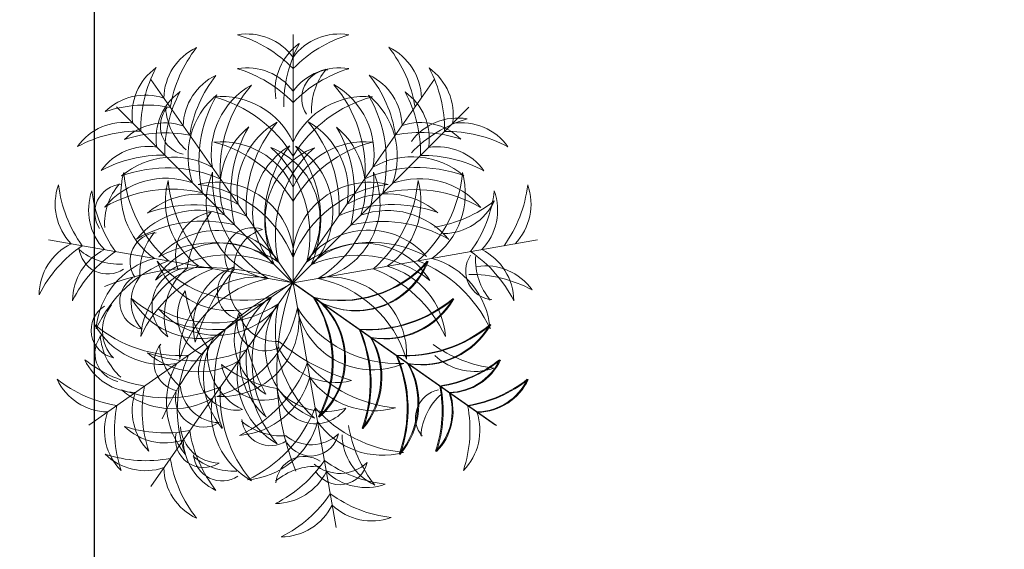
# Model space of a CAD drawing. Units: inches. Extents: x -48 to 50072, y 0 to 21068.
# Tile 10 of 75: x 212 to 263, y 278 to 305. Entities that reach past the tile are written whole.
import ezdxf

# ---------------------------------------------------------------- set-up
doc = ezdxf.new("R2010")
doc.units = ezdxf.units.IN
doc.header["$MEASUREMENT"] = 0
doc.layers.add('A-ANNO-DIMS', color=2, linetype='Continuous', lineweight=18)
doc.layers.add('L-PLNT', color=94, linetype='Continuous', lineweight=13)
doc.styles.get("Standard").update_dxf_attribs({"font": 'arial.ttf'})
doc.dimstyles.get("Standard").update_dxf_attribs({"dimtxt": 8, "dimasz": 0.18, "dimexe": 0.18, "dimexo": 0.0625, "dimgap": 0.09, "dimtad": 0, "dimtih": 1, "dimtoh": 1, "dimdec": 1, "dimzin": 0, "dimdsep": 46, "dimlunit": 4, "dimtxsty": 'Standard', "dimblk": 'ARCHTICK', "dimcen": 0.09, "dimadec": 0, "dimazin": 0, "dimtfac": 1, "dimtdec": 1, "dimtofl": 0, "dimtmove": 0, "dimatfit": 3, "dimldrblk": 'ARCHTICK', "dimfxl": 1, "dimtolj": 1, "dimtzin": 0, "dimarcsym": 0})

# ---------------------------------------------------------------- blocks, each defined once
blk = doc.blocks.new('A$C5D061C3B')
for p, q in [((3.377, 6.679), (3.377, 3.377)), ((1.483, 6.082), (3.377, 3.377)), ((5.259, 6.086), (3.365, 3.381)), ((1.03, 5.716), (3.365, 3.381)), ((5.712, 5.712), (3.377, 3.377)), ((0.125, 3.951), (3.377, 3.377)), ((6.629, 3.951), (3.377, 3.377)), ((0.66, 1.487), (3.365, 3.381)), ((1.483, 0.672), (3.377, 3.377)), ((6.07, 1.487), (3.365, 3.381)), ((3.951, 0.125), (3.377, 3.377)), ((6.082, 1.483), (3.377, 3.377))]:
    blk.add_line(p, q)
for centre, radius, start, end in [((2.763, 5.924), 0.762, 36.29, 99.6243), ((3.991, 5.924), 0.762, 80.3757, 143.71), ((2.145, 5.032), 1.715, 44.0763, 73.3794), ((3.901, 5.939), 0.762, 125.3757, 188.71), ((4.969, 5.745), 1.715, 151.6206, 180.9237), ((4.61, 5.032), 1.715, 106.6206, 135.9237), ((2.419, 5.816), 0.762, 115.3757, 178.71), ((3.438, 5.44), 1.715, 141.6206, 170.9237), ((3.305, 5.444), 1.715, 9.0763, 38.3794), ((4.323, 5.82), 0.762, 1.29, 64.6243), ((1.998, 5.617), 0.762, 125.3757, 188.71), ((3.066, 5.423), 1.715, 151.6206, 180.9237), ((2.763, 5.474), 0.762, 36.29, 99.6243), ((2.145, 4.581), 1.715, 44.0763, 73.3794), ((3.991, 5.474), 0.762, 80.3757, 143.71), ((4.61, 4.581), 1.715, 106.6206, 135.9237), ((3.871, 5.832), 0.38, 94.742, 213.7475), ((4.447, 5.681), 0.826, 139.618, 183.2106), ((4.744, 5.613), 0.762, 351.29, 54.6243), ((3.676, 5.419), 1.715, 359.0763, 28.3794), ((2.678, 5.447), 0.762, 115.3757, 178.71), ((3.696, 5.07), 1.715, 141.6206, 170.9237), ((4.064, 5.451), 0.762, 1.29, 64.6243), ((3.046, 5.075), 1.715, 9.0763, 38.3794), ((2.317, 5.298), 0.762, 125.3757, 188.71), ((3.385, 5.104), 1.715, 151.6206, 180.9237), ((3.344, 5.089), 1.056, 119.6063, 189.7511), ((4.177, 4.869), 1.77, 139.9634, 183.6288), ((3.398, 5.094), 1.056, 350.2489, 60.3937), ((2.565, 4.873), 1.77, 356.3712, 40.0366), ((3.357, 5.1), 1.715, 359.0763, 28.3794), ((4.425, 5.294), 0.762, 351.29, 54.6243), ((1.413, 5.111), 0.762, 71.29, 134.6243), ((3.035, 5.062), 1.056, 129.6063, 199.7511), ((3.894, 4.989), 1.77, 149.9634, 193.6288), ((2.422, 4.799), 1.056, 25.2489, 95.3937), ((1.866, 4.14), 1.77, 31.3712, 75.0366), ((4.332, 4.799), 1.056, 84.6063, 154.7511), ((4.888, 4.14), 1.77, 104.9634, 148.6288), ((2.848, 4.985), 1.77, 346.3712, 30.0366), ((3.707, 5.058), 1.056, 340.2489, 50.3937), ((1.419, 4.026), 1.715, 79.0763, 108.3794), ((1.991, 5.462), 0.38, 139.742, 258.7475), ((2.505, 5.763), 0.826, 184.618, 228.2106), ((1.13, 4.748), 0.762, 81.29, 144.6243), ((1.671, 4.742), 0.762, 71.29, 134.6243), ((3.688, 4.597), 1.056, 119.6063, 189.7511), ((4.522, 4.377), 1.77, 139.9634, 183.6288), ((2.221, 4.381), 1.77, 356.3712, 40.0366), ((3.054, 4.602), 1.056, 350.2489, 60.3937), ((5.071, 4.746), 0.762, 45.3757, 108.71), ((5.564, 4.807), 0.762, 80.3757, 143.71), ((6.182, 3.914), 1.715, 106.6206, 135.9237), ((5.613, 4.744), 0.762, 35.3757, 98.71), ((1.324, 3.68), 1.715, 89.0763, 118.3794), ((1.677, 3.657), 1.715, 79.0763, 108.3794), ((3.46, 4.637), 1.056, 129.6063, 199.7511), ((4.319, 4.565), 1.77, 149.9634, 193.6288), ((3.283, 4.633), 1.056, 340.2489, 50.3937), ((2.424, 4.56), 1.77, 346.3712, 30.0366), ((5.065, 3.661), 1.715, 71.6206, 100.9237), ((5.419, 3.676), 1.715, 61.6206, 90.9237), ((2.422, 4.198), 1.056, 25.2489, 95.3937), ((1.866, 3.54), 1.77, 31.3712, 75.0366), ((4.332, 4.198), 1.056, 84.6063, 154.7511), ((4.888, 3.54), 1.77, 104.9634, 148.6288), ((1.448, 4.43), 0.762, 81.29, 144.6243), ((3.868, 4.321), 1.029, 121.3654, 221.5741), ((4.556, 4.237), 1.557, 141.8122, 203.3335), ((4.035, 4.215), 1.029, 111.3654, 211.5741), ((2.707, 4.219), 1.029, 328.4259, 68.6346), ((2.044, 4.017), 1.557, 346.6665, 48.1878), ((4.698, 4.013), 1.557, 131.8122, 193.3335), ((2.187, 4.233), 1.557, 336.6665, 38.1878), ((2.875, 4.316), 1.029, 318.4259, 58.6346), ((5.294, 4.425), 0.762, 35.3757, 98.71), ((1.642, 3.362), 1.715, 89.0763, 118.3794), ((1.78, 3.994), 1.056, 60.2489, 130.3937), ((4.963, 3.998), 1.056, 49.6063, 119.7511), ((5.1, 3.357), 1.715, 61.6206, 90.9237), ((1.702, 3.136), 1.77, 66.3712, 110.0366), ((3.25, 4.435), 1.029, 156.3654, 256.5741), ((3.862, 4.761), 1.557, 176.8122, 238.3335), ((2.893, 4.761), 1.557, 301.6665, 3.1878), ((3.504, 4.435), 1.029, 283.4259, 23.6346), ((5.04, 3.14), 1.77, 69.9634, 113.6288), ((1.685, 3.712), 1.056, 70.2489, 140.3937), ((2.143, 4.564), 1.056, 164.6063, 234.7511), ((2.888, 4.998), 1.77, 184.9634, 228.6288), ((2.734, 4.46), 1.056, 164.6063, 234.7511), ((3.48, 4.893), 1.77, 184.9634, 228.6288), ((2.358, 3.686), 1.029, 3.4259, 103.6346), ((4.397, 3.686), 1.029, 76.3654, 176.5741), ((3.275, 4.893), 1.77, 311.3712, 355.0366), ((4.02, 4.46), 1.056, 305.2489, 15.3937), ((5.058, 3.707), 1.056, 39.6063, 109.7511), ((3.866, 4.998), 1.77, 311.3712, 355.0366), ((4.611, 4.564), 1.056, 305.2489, 15.3937), ((0.975, 4.424), 0.762, 160.3757, 223.71), ((1.962, 4.878), 1.715, 186.6206, 215.9237), ((1.419, 4.346), 0.762, 160.3757, 223.71), ((2.405, 4.8), 1.715, 186.6206, 215.9237), ((1.12, 4.31), 0.38, 94.742, 213.7475), ((1.696, 4.159), 0.826, 139.618, 183.2106), ((1.757, 2.853), 1.77, 76.3712, 120.0366), ((1.93, 3.14), 1.557, 21.6665, 83.1878), ((4.824, 3.14), 1.557, 96.8122, 158.3335), ((4.985, 2.848), 1.77, 59.9634, 103.6288), ((4.349, 4.8), 1.715, 324.0763, 353.3794), ((5.335, 4.346), 0.762, 316.29, 19.6243), ((4.793, 4.878), 1.715, 324.0763, 353.3794), ((5.779, 4.424), 0.762, 316.29, 19.6243), ((2.124, 3.502), 1.056, 60.2489, 130.3937), ((4.618, 3.506), 1.056, 49.6063, 119.7511), ((4.988, 5.812), 1.715, 279.0763, 308.3794), ((5.365, 4.794), 0.762, 271.29, 334.6243), ((2.109, 3.287), 1.056, 70.2489, 140.3937), ((2.046, 2.644), 1.77, 66.3712, 110.0366), ((4.696, 2.648), 1.77, 69.9634, 113.6288), ((4.633, 3.283), 1.056, 39.6063, 109.7511), ((2.182, 2.428), 1.77, 76.3712, 120.0366), ((2.387, 3.752), 0.574, 99.9865, 199.4034), ((3.599, 3.314), 1.651, 142.5759, 170.8942), ((4.56, 2.424), 1.77, 59.9634, 103.6288), ((2.365, 3.045), 1.029, 38.4259, 138.6346), ((2.84, 3.739), 0.372, 69.2257, 210.1279), ((3.109, 3.59), 0.515, 105.4398, 183.6694), ((4.377, 3.05), 1.029, 41.3654, 141.5741), ((1.588, 3.666), 0.38, 94.742, 213.7475), ((2.165, 3.515), 0.826, 139.618, 183.2106), ((0.762, 3.214), 0.762, 116.29, 179.6243), ((1.534, 2.451), 1.715, 124.0763, 153.3794), ((1.206, 3.136), 0.762, 116.29, 179.6243), ((1.062, 4.452), 0.826, 229.618, 273.2106), ((0.91, 3.875), 0.38, 184.742, 303.7475), ((2.426, 2.879), 1.029, 48.4259, 148.6346), ((2.328, 2.353), 1.557, 56.6665, 118.1878), ((4.414, 2.358), 1.557, 61.8122, 123.3335), ((4.316, 2.875), 1.029, 31.3654, 131.5741), ((5.549, 3.136), 0.762, 0.3757, 63.71), ((1.977, 2.373), 1.715, 124.0763, 153.3794), ((1.811, 2.684), 1.056, 105.2489, 175.3937), ((2.363, 2.022), 1.77, 111.3712, 155.0366), ((2.51, 2.191), 1.557, 66.6665, 128.1878), ((4.233, 2.187), 1.557, 51.8122, 113.3335), ((4.391, 2.022), 1.77, 24.9634, 68.6288), ((4.943, 2.684), 1.056, 4.6063, 74.7511), ((6.053, 3.533), 0.38, 146.2525, 265.258), ((4.777, 2.373), 1.715, 26.6206, 55.9237), ((6.629, 3.684), 0.826, 176.7894, 220.382), ((2.185, 0.015), 3.567, 70.4772, 111.6585), ((2.403, 2.58), 1.056, 105.2489, 175.3937), ((2.955, 1.917), 1.77, 111.3712, 155.0366), ((2.007, 3.071), 0.506, 93.8744, 233.9763), ((2.729, 4.702), 1.557, 221.8122, 283.3335), ((2.527, 4.039), 1.029, 201.3654, 301.5741), ((2.489, 2.932), 0.825, 128.7536, 199.097), ((2.903, 2.8), 0.855, 116.4477, 194.3672), ((4.744, 1.779), 2.789, 140.4007, 163.139), ((2.741, 3.253), 0.372, 114.2257, 255.1279), ((3.037, 3.338), 0.515, 150.4398, 228.6694), ((4.001, 4.702), 1.557, 256.6665, 318.1878), ((4.013, 4.698), 1.557, 256.6665, 318.1878), ((4.203, 4.039), 1.029, 238.4259, 338.6346), ((4.215, 4.035), 1.029, 238.4259, 338.6346), ((3.799, 1.917), 1.77, 24.9634, 68.6288), ((4.352, 2.58), 1.056, 4.6063, 74.7511), ((5.935, 2.842), 0.762, 35.3757, 98.71), ((1.447, 3.129), 0.376, 122.0577, 257.8533), ((1.751, 3.126), 0.529, 140.1845, 223.654), ((2.896, 2.427), 1.029, 83.4259, 183.6346), ((3.359, 1.911), 1.557, 101.6665, 163.1878), ((3.395, 1.911), 1.557, 16.8122, 78.3335), ((3.858, 2.427), 1.029, 356.3654, 96.5741), ((5.741, 1.774), 1.715, 61.6206, 90.9237), ((4.912, 0.157), 3.567, 115.4772, 156.6585), ((6.727, 2.189), 3.567, 160.4772, 201.6585), ((2.145, 3.693), 1.056, 209.6063, 279.7511), ((2.365, 4.526), 1.77, 229.9634, 273.6288), ((2.412, 2.943), 0.574, 144.9865, 244.4034), ((3.578, 3.49), 1.651, 187.5759, 215.8942), ((3.697, 2.369), 1.029, 128.4259, 228.6346), ((4.389, 2.332), 1.557, 146.6665, 208.1878), ((2.341, 2.332), 1.557, 331.8122, 33.3335), ((2.353, 2.328), 1.557, 331.8122, 33.3335), ((3.033, 2.369), 1.029, 311.3654, 51.5741), ((3.045, 2.365), 1.029, 311.3654, 51.5741), ((4.365, 4.526), 1.77, 266.3712, 310.0366), ((4.377, 4.522), 1.77, 266.3712, 310.0366), ((4.585, 3.693), 1.056, 260.2489, 330.3937), ((4.597, 3.688), 1.056, 260.2489, 330.3937), ((1.067, 2.749), 0.376, 122.0577, 257.8533), ((1.37, 2.745), 0.529, 140.1845, 223.654), ((2.328, 4.401), 1.557, 241.8122, 303.3335), ((2.365, 3.709), 1.029, 221.3654, 321.5741), ((1.911, 3.359), 1.557, 286.8122, 348.3335), ((2.427, 2.896), 1.029, 266.3654, 6.5741), ((4.035, 2.539), 1.029, 148.4259, 248.6346), ((4.698, 2.741), 1.557, 166.6665, 228.1878), ((4.761, 3.862), 1.557, 211.6665, 273.1878), ((3.45, 2.634), 0.855, 161.4477, 239.3672), ((3.003, 2.844), 0.372, 159.2257, 300.1279), ((3.152, 3.113), 0.515, 195.4398, 273.6694), ((5.474, 3.214), 2.789, 185.4007, 208.139), ((4.435, 3.25), 1.029, 193.4259, 293.6346), ((1.873, 4.181), 1.77, 229.9634, 273.6288), ((1.653, 3.348), 1.056, 209.6063, 279.7511), ((4.099, 2.051), 1.77, 156.3712, 200.0366), ((2.632, 2.051), 1.77, 339.9634, 23.6288), ((2.644, 2.046), 1.77, 339.9634, 23.6288), ((4.857, 4.181), 1.77, 266.3712, 310.0366), ((4.869, 4.177), 1.77, 266.3712, 310.0366), ((5.077, 3.348), 1.056, 260.2489, 330.3937), ((5.089, 3.344), 1.056, 260.2489, 330.3937), ((1.122, 2.441), 0.38, 139.742, 258.7475), ((1.636, 2.741), 0.826, 184.618, 228.2106), ((3.24, 2.128), 1.056, 150.2489, 220.3937), ((3.49, 2.128), 1.056, 319.6063, 29.7511), ((3.502, 2.124), 1.056, 319.6063, 29.7511), ((2.046, 4.111), 1.77, 249.9634, 293.6288), ((1.908, 2.317), 0.38, 139.742, 258.7475), ((2.422, 2.617), 0.826, 184.618, 228.2106), ((2.624, 2.192), 0.506, 138.8744, 278.9763), ((3.064, 2.435), 0.825, 173.7536, 244.097), ((4.522, 2.378), 1.77, 176.3712, 220.0366), ((3.942, 2.908), 0.855, 206.4477, 284.3672), ((4.963, 4.749), 2.789, 230.4007, 253.139), ((6.244, 3.948), 1.715, 234.0763, 263.3794), ((2.124, 3.252), 1.056, 229.6063, 299.7511), ((3.607, 1.706), 1.77, 156.3712, 200.0366), ((3.124, 1.706), 1.77, 339.9634, 23.6288), ((3.136, 1.702), 1.77, 339.9634, 23.6288), ((5.79, 2.962), 0.762, 226.29, 289.6243), ((1.672, 3.7), 1.715, 231.6206, 260.9237), ((1.295, 2.682), 0.762, 205.3757, 268.71), ((2.748, 1.784), 1.056, 150.2489, 220.3937), ((3.428, 3.603), 1.651, 232.5759, 260.8942), ((2.99, 2.391), 0.574, 189.9865, 289.4034), ((3.688, 2.157), 1.056, 170.2489, 240.3937), ((1.917, 2.955), 1.77, 294.9634, 338.6288), ((4.893, 3.48), 1.77, 221.3712, 265.0366), ((3.982, 1.784), 1.056, 319.6063, 29.7511), ((3.994, 1.78), 1.056, 319.6063, 29.7511), ((5.058, 3.7), 1.715, 279.0763, 308.3794), ((5.07, 3.696), 1.715, 279.0763, 308.3794), ((5.435, 2.682), 0.762, 271.29, 334.6243), ((5.447, 2.678), 0.762, 271.29, 334.6243), ((0.926, 2.424), 0.762, 205.3757, 268.71), ((1.303, 3.442), 1.715, 231.6206, 260.9237), ((2.58, 2.403), 1.056, 274.6063, 344.7511), ((4.46, 2.734), 1.056, 215.2489, 285.3937), ((5.427, 3.442), 1.715, 279.0763, 308.3794), ((5.804, 2.424), 0.762, 271.29, 334.6243), ((1.702, 3.619), 1.77, 249.9634, 293.6288), ((3.086, 1.681), 1.715, 169.0763, 198.3794), ((2.405, 2.049), 0.529, 185.1845, 268.654), ((4.177, 1.886), 1.77, 176.3712, 220.0366), ((3.81, 2.493), 0.825, 218.7536, 289.097), ((3.671, 2.011), 0.506, 183.8744, 323.9763), ((3.645, 1.681), 1.715, 341.6206, 10.9237), ((3.657, 1.677), 1.715, 341.6206, 10.9237), ((5.44, 3.438), 1.715, 279.0763, 308.3794), ((5.816, 2.419), 0.762, 271.29, 334.6243), ((1.78, 2.76), 1.056, 229.6063, 299.7511), ((2, 1.676), 0.762, 161.29, 224.6243), ((2.188, 1.837), 0.376, 167.0577, 302.8533), ((3.344, 1.665), 1.056, 170.2489, 240.3937), ((5.385, 1.584), 0.38, 101.2525, 220.258), ((5.899, 1.283), 0.826, 131.7894, 175.382), ((4.73, 1.676), 0.762, 315.3757, 18.71), ((4.742, 1.671), 0.762, 315.3757, 18.71), ((2.717, 1.423), 1.715, 169.0763, 198.3794), ((2.022, 2.363), 1.77, 294.9634, 338.6288), ((4.998, 2.888), 1.77, 221.3712, 265.0366), ((4.014, 1.423), 1.715, 341.6206, 10.9237), ((1.631, 1.417), 0.762, 161.29, 224.6243), ((5.099, 1.417), 0.762, 315.3757, 18.71), ((1.671, 2.012), 0.762, 225.3757, 288.71), ((1.677, 3.098), 1.715, 251.6206, 280.9237), ((2.405, 1.511), 0.529, 185.1845, 268.654), ((3.227, 2.169), 0.826, 229.618, 273.2106), ((3.076, 1.593), 0.38, 184.742, 303.7475), ((2.684, 1.811), 1.056, 274.6063, 344.7511), ((4.564, 2.143), 1.056, 215.2489, 285.3937), ((5.808, 1.754), 1.715, 189.0763, 218.3794), ((2.188, 1.299), 0.376, 167.0577, 302.8533), ((3.696, 1.684), 1.715, 189.0763, 218.3794), ((3.616, 1.755), 0.529, 230.1845, 313.654), ((3.613, 1.452), 0.376, 212.0577, 347.8533), ((4.79, 1.377), 0.762, 181.29, 244.6243), ((2.678, 1.307), 0.762, 181.29, 244.6243), ((1.419, 2.729), 1.715, 251.6206, 280.9237), ((1.413, 1.643), 0.762, 225.3757, 288.71), ((2.583, 1.701), 0.826, 229.618, 273.2106), ((2.432, 1.124), 0.38, 184.742, 303.7475), ((3.528, 0.69), 0.38, 56.2525, 175.258), ((2.419, 0.938), 0.762, 181.29, 244.6243), ((3.438, 1.315), 1.715, 189.0763, 218.3794), ((2.373, 1.977), 1.715, 296.6206, 325.9237), ((3.68, 0.113), 0.826, 86.7894, 130.382), ((3.997, 1.374), 0.529, 230.1845, 313.654), ((3.994, 1.071), 0.376, 212.0577, 347.8533), ((4.8, 2.405), 1.715, 234.0763, 263.3794), ((3.136, 1.206), 0.762, 270.3757, 333.71), ((4.346, 1.419), 0.762, 226.29, 289.6243), ((2.451, 1.534), 1.715, 296.6206, 325.9237), ((4.878, 1.962), 1.715, 234.0763, 263.3794), ((3.214, 0.762), 0.762, 270.3757, 333.71), ((4.424, 0.975), 0.762, 226.29, 289.6243)]:
    blk.add_arc(centre, radius, start, end)
blk = doc.blocks.new('_ArchTick')
at = {"color": 0, "linetype": 'ByBlock', "const_width": 0.15}
blk.add_lwpolyline([(-0.5, -0.5), (0.5, 0.5)], dxfattribs=at)
blk = doc.blocks.new('*D116')
at = {"layer": 'A-ANNO-DIMS', "color": 0, "lineweight": -2, "transparency": 16777216}
for p, q in [((18.017, 677.712), (18.017, 165.945)), ((216.017, 677.712), (216.017, 165.945)), ((18.017, 166.125), (108.458, 166.125)), ((216.017, 166.125), (125.576, 166.125))]:
    blk.add_line(p, q, dxfattribs=at)
at = {"layer": 'Defpoints', "color": 0, "transparency": 16777216}
for p in [(18.017, 677.775), (216.017, 677.775), (216.017, 166.125)]:
    blk.add_point(p, dxfattribs=at)
at = {"layer": 'A-ANNO-DIMS', "color": 0, "lineweight": -2, "transparency": 16777216, "xscale": 0.18, "yscale": 0.18, "zscale": 0.18, "rotation": 180}
blk.add_blockref('_ArchTick', (18.017, 166.125), dxfattribs=at)
at = {"layer": 'A-ANNO-DIMS', "color": 0, "lineweight": -2, "transparency": 16777216, "xscale": 0.18, "yscale": 0.18, "zscale": 0.18}
blk.add_blockref('_ArchTick', (216.017, 166.125), dxfattribs=at)
at = {"layer": 'A-ANNO-DIMS', "color": 0, "transparency": 16777216, "insert": (117.017, 166.125), "char_height": 8, "attachment_point": 5}
blk.add_mtext('\\A1;198', dxfattribs=at)
blk = doc.blocks.new('*D117')
at = {"layer": 'A-ANNO-DIMS', "color": 0, "lineweight": -2, "transparency": 16777216}
for p, q in [((216.017, 488.712), (216.017, 165.945)), ((297.017, 488.712), (297.017, 165.945)), ((216.017, 166.125), (251.464, 166.125)), ((297.017, 166.125), (261.57, 166.125))]:
    blk.add_line(p, q, dxfattribs=at)
at = {"layer": 'Defpoints', "color": 0, "transparency": 16777216}
for p in [(216.017, 488.775), (297.017, 488.775), (297.017, 166.125)]:
    blk.add_point(p, dxfattribs=at)
at = {"layer": 'A-ANNO-DIMS', "color": 0, "lineweight": -2, "transparency": 16777216, "xscale": 0.18, "yscale": 0.18, "zscale": 0.18, "rotation": 180}
blk.add_blockref('_ArchTick', (216.017, 166.125), dxfattribs=at)
at = {"layer": 'A-ANNO-DIMS', "color": 0, "lineweight": -2, "transparency": 16777216, "xscale": 0.18, "yscale": 0.18, "zscale": 0.18}
blk.add_blockref('_ArchTick', (297.017, 166.125), dxfattribs=at)
at = {"layer": 'A-ANNO-DIMS', "color": 0, "transparency": 16777216, "insert": (256.517, 166.125), "char_height": 8, "attachment_point": 5}
blk.add_mtext('\\A1;81', dxfattribs=at)

msp = doc.modelspace()

# ---------------------------------------------------------------- block references
at = {"layer": 'L-PLNT', "xscale": 3.862191520948588, "yscale": 3.862191520948588, "zscale": 3.862191520948588}
msp.add_blockref('A$C5D061C3B', (213.183, 278.619), dxfattribs=at)

# ---------------------------------------------------------------- dimensions: what is measured, and where the dimension line sits
at = {"layer": 'A-ANNO-DIMS'}
for base, p1, p2, picture, middle in [((216.017, 166.125), (18.017, 677.775), (216.017, 677.775), '*D116', (117.017, 166.125)), ((297.017, 166.125), (216.017, 488.775), (297.017, 488.775), '*D117', (256.517, 166.125))]:
    dim = msp.add_linear_dim(base=base, p1=p1, p2=p2, dimstyle='Standard', override={"dimdec": 0, "dimlfac": 1, "dimrnd": 0, "dimzin": 0, "dimdsep": 46, "dimlunit": 2}, dxfattribs=at)
    dim.commit()
    dim.dimension.update_dxf_attribs({"geometry": picture, "text_midpoint": middle})

doc.saveas('drawing.dxf')
